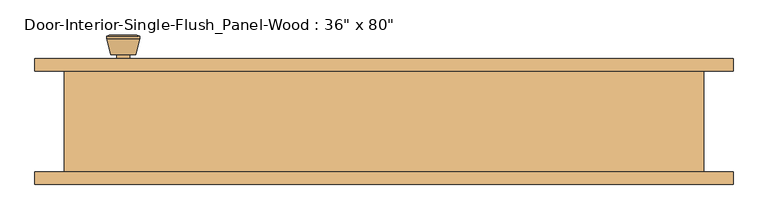
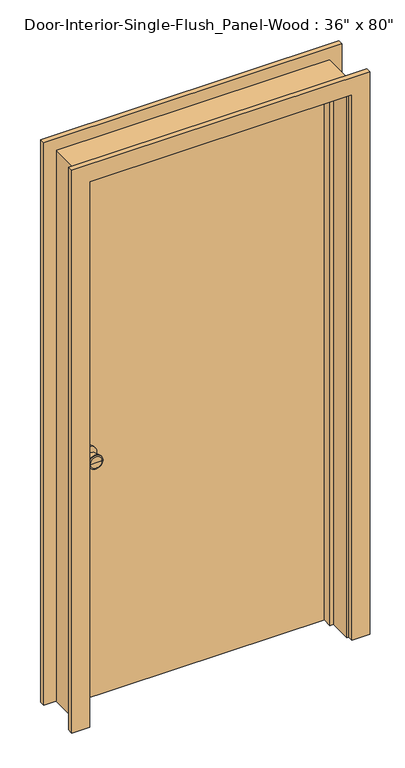
"""IFC4 building model written with IfcOpenShell, lengths in millimetres: door geometry."""

from ifc_helpers import new_model, si_unit, point, frame, frame_2d, origin, origin_with_axes, place, context, project, spatial, polyline, circle_curve, trimmed, segment, composite_curve, outline, extrude, faceted_brep, source, transform, mapped, element, save
from ifc_brep_helpers import plane_surface, cylinder_surface, revolved_surface, advanced_brep


def door_2171c7d8(model_context):
    return source(origin(), model_context, "Body", "SolidModel", [
        advanced_brep(
        [(-393.7, 32.1, 914.4), (-383.7, 32.1, 914.4), (-403.7, 32.1, 914.4), (-373.2241324, -16.9, 914.4), (-393.7, -16.9, 914.4), (-414.1758676, -16.9, 914.4), (-368.7, -15.0721319, 914.4), (-418.7, -15.0721319, 914.4), (-368.7, -11.6084537, 914.4), (-418.7, -11.6084537, 914.4), (-375.063764, 13.1, 914.4), (-412.336236, 13.1, 914.4), (-383.7, 13.1, 914.4), (-403.7, 13.1, 914.4)],
        [
            (0, 1),
            (1, 2, circle_curve(frame((-393.7, 32.1, 914.4), z_axis=(0.0, 1.0, 0.0), x_axis=(-1.0, 0.0, 0.0)), 10.0)),
            (2, 0),
            (2, 1, circle_curve(frame((-393.7, 32.1, 914.4), z_axis=(0.0, 1.0, 0.0), x_axis=(-1.0, 0.0, 0.0)), 10.0)),
            (3, 4),
            (4, 5),
            (5, 3, circle_curve(frame((-393.7, -16.9, 914.4), z_axis=(0.0, -1.0, 0.0), x_axis=(-1.0, 0.0, 0.0)), 20.4758676)),
            (3, 5, circle_curve(frame((-393.7, -16.9, 914.4), z_axis=(0.0, -1.0, 0.0), x_axis=(-1.0, 0.0, 0.0)), 20.4758676)),
            (6, 3),
            (5, 7),
            (7, 6, circle_curve(frame((-393.7, -15.0721319, 914.4), z_axis=(0.0, -1.0, 0.0), x_axis=(-1.0, 0.0, 0.0)), 25.0)),
            (6, 7, circle_curve(frame((-393.7, -15.0721319, 914.4), z_axis=(0.0, -1.0, 0.0), x_axis=(-1.0, 0.0, 0.0)), 25.0)),
            (8, 6),
            (7, 9),
            (9, 8, circle_curve(frame((-393.7, -11.6084537, 914.4), z_axis=(0.0, -1.0, 0.0), x_axis=(-1.0, 0.0, 0.0)), 25.0)),
            (8, 9, circle_curve(frame((-393.7, -11.6084537, 914.4), z_axis=(0.0, -1.0, 0.0), x_axis=(-1.0, 0.0, 0.0)), 25.0)),
            (10, 8),
            (9, 11),
            (11, 10, circle_curve(frame((-393.7, 13.1, 914.4), z_axis=(0.0, -1.0, 0.0), x_axis=(-1.0, 0.0, 0.0)), 18.636236)),
            (10, 11, circle_curve(frame((-393.7, 13.1, 914.4), z_axis=(0.0, -1.0, 0.0), x_axis=(-1.0, 0.0, 0.0)), 18.636236)),
            (12, 10),
            (11, 13),
            (13, 12, circle_curve(frame((-393.7, 13.1, 914.4), z_axis=(0.0, -1.0, 0.0), x_axis=(-1.0, 0.0, 0.0)), 10.0)),
            (12, 13, circle_curve(frame((-393.7, 13.1, 914.4), z_axis=(0.0, -1.0, 0.0), x_axis=(-1.0, 0.0, 0.0)), 10.0)),
            (1, 12),
            (13, 2),
        ],
        [
            plane_surface(frame((-393.7, 32.1, 914.4), z_axis=(0.0, 1.0, 0.0), x_axis=(-1.0, 0.0, 0.0))),
            plane_surface(frame((-393.7, -16.9, 914.4), z_axis=(0.0, -1.0, 0.0), x_axis=(-1.0, 0.0, 0.0))),
            revolved_surface(polyline([(-414.1758676, -16.9, 914.4), (-418.7, -15.0721319, 914.4)]), (-393.7, 32.1, 914.4), (0.0, 1.0, 0.0)),
            cylinder_surface(frame((-393.7, 32.1, 914.4), z_axis=(0.0, 1.0, 0.0), x_axis=(-1.0, 0.0, 0.0)), 25.0),
            revolved_surface(polyline([(-418.7, -11.6084537, 914.4), (-412.336236, 13.1, 914.4)]), (-393.7, 32.1, 914.4), (0.0, 1.0, 0.0)),
            plane_surface(frame((-393.7, 13.1, 914.4), z_axis=(0.0, 1.0, 0.0), x_axis=(-1.0, 0.0, 0.0))),
            cylinder_surface(frame((-393.7, 32.1, 914.4), z_axis=(0.0, 1.0, 0.0), x_axis=(-1.0, 0.0, 0.0)), 10.0),
        ],
        [
            (0, [[1, 2, 3]]),
            (0, [[-3, 4, -1]]),
            (1, [[5, 6, 7]]),
            (1, [[-6, -5, 8]]),
            (2, [[9, -7, 10, 11]]),
            (2, [[-10, -8, -9, 12]]),
            (3, [[13, -11, 14, 15]]),
            (3, [[-14, -12, -13, 16]]),
            (4, [[17, -15, 18, 19]]),
            (4, [[-18, -16, -17, 20]]),
            (5, [[21, -19, 22, 23]]),
            (5, [[-22, -20, -21, 24]]),
            (6, [[25, -23, 26, -2]]),
            (6, [[-26, -24, -25, -4]]),
        ],
    ),
        extrude(outline(composite_curve([segment(trimmed(circle_curve(frame_2d((914.4, -393.7)), 30.0), [point((914.4, -423.7))], [point((914.4, -363.7))], False, "CARTESIAN"), True, "CONTINUOUS"), segment(trimmed(circle_curve(frame_2d((914.4, -393.7)), 30.0), [point((914.4, -363.7))], [point((914.4, -423.7))], False, "CARTESIAN"), True, "CONTINUOUS")], self_intersect=False)), frame((0.0, 32.1, 0.0), z_axis=(0.0, 1.0, 0.0), x_axis=(0.0, 0.0, 1.0)), (0.0, 0.0, 1.0), 6.0),
        advanced_brep(
        [(-393.7, 79.025, 914.4), (-403.7, 79.025, 914.4), (-383.7, 79.025, 914.4), (-373.2241324, 128.025, 914.4), (-414.1758676, 128.025, 914.4), (-393.7, 128.025, 914.4), (-368.7, 126.1971319, 914.4), (-418.7, 126.1971319, 914.4), (-368.7, 122.7334537, 914.4), (-418.7, 122.7334537, 914.4), (-375.063764, 98.025, 914.4), (-412.336236, 98.025, 914.4), (-383.7, 98.025, 914.4), (-403.7, 98.025, 914.4)],
        [
            (0, 1),
            (1, 2, circle_curve(frame((-393.7, 79.025, 914.4), z_axis=(0.0, -1.0, 0.0), x_axis=(-1.0, 0.0, 0.0)), 10.0)),
            (2, 0),
            (2, 1, circle_curve(frame((-393.7, 79.025, 914.4), z_axis=(0.0, -1.0, 0.0), x_axis=(-1.0, 0.0, 0.0)), 10.0)),
            (3, 4, circle_curve(frame((-393.7, 128.025, 914.4), z_axis=(0.0, 1.0, 0.0), x_axis=(-1.0, 0.0, 0.0)), 20.4758676)),
            (4, 5),
            (5, 3),
            (4, 3, circle_curve(frame((-393.7, 128.025, 914.4), z_axis=(0.0, 1.0, 0.0), x_axis=(-1.0, 0.0, 0.0)), 20.4758676)),
            (6, 7, circle_curve(frame((-393.7, 126.1971319, 914.4), z_axis=(0.0, 1.0, 0.0), x_axis=(-1.0, 0.0, 0.0)), 25.0)),
            (7, 4),
            (3, 6),
            (7, 6, circle_curve(frame((-393.7, 126.1971319, 914.4), z_axis=(0.0, 1.0, 0.0), x_axis=(-1.0, 0.0, 0.0)), 25.0)),
            (8, 9, circle_curve(frame((-393.7, 122.7334537, 914.4), z_axis=(0.0, 1.0, 0.0), x_axis=(-1.0, 0.0, 0.0)), 25.0)),
            (9, 7),
            (6, 8),
            (9, 8, circle_curve(frame((-393.7, 122.7334537, 914.4), z_axis=(0.0, 1.0, 0.0), x_axis=(-1.0, 0.0, 0.0)), 25.0)),
            (10, 11, circle_curve(frame((-393.7, 98.025, 914.4), z_axis=(0.0, 1.0, 0.0), x_axis=(-1.0, 0.0, 0.0)), 18.636236)),
            (11, 9),
            (8, 10),
            (11, 10, circle_curve(frame((-393.7, 98.025, 914.4), z_axis=(0.0, 1.0, 0.0), x_axis=(-1.0, 0.0, 0.0)), 18.636236)),
            (12, 13, circle_curve(frame((-393.7, 98.025, 914.4), z_axis=(0.0, 1.0, 0.0), x_axis=(-1.0, 0.0, 0.0)), 10.0)),
            (13, 11),
            (10, 12),
            (13, 12, circle_curve(frame((-393.7, 98.025, 914.4), z_axis=(0.0, 1.0, 0.0), x_axis=(-1.0, 0.0, 0.0)), 10.0)),
            (1, 13),
            (12, 2),
        ],
        [
            plane_surface(frame((-393.7, 79.025, 914.4), z_axis=(0.0, -1.0, 0.0), x_axis=(-1.0, 0.0, 0.0))),
            plane_surface(frame((-393.7, 128.025, 914.4), z_axis=(0.0, 1.0, 0.0), x_axis=(-1.0, 0.0, 0.0))),
            revolved_surface(polyline([(-414.1758676, 128.025, 914.4), (-418.7, 126.1971319, 914.4)]), (-393.7, 79.025, 914.4), (0.0, -1.0, 0.0)),
            cylinder_surface(frame((-393.7, 79.025, 914.4), z_axis=(0.0, -1.0, 0.0), x_axis=(-1.0, 0.0, 0.0)), 25.0),
            revolved_surface(polyline([(-418.7, 122.7334537, 914.4), (-412.336236, 98.025, 914.4)]), (-393.7, 79.025, 914.4), (0.0, -1.0, 0.0)),
            plane_surface(frame((-393.7, 98.025, 914.4), z_axis=(0.0, -1.0, 0.0), x_axis=(-1.0, 0.0, 0.0))),
            cylinder_surface(frame((-393.7, 79.025, 914.4), z_axis=(0.0, -1.0, 0.0), x_axis=(-1.0, 0.0, 0.0)), 10.0),
        ],
        [
            (0, [[1, 2, 3]]),
            (0, [[-3, 4, -1]]),
            (1, [[5, 6, 7]]),
            (1, [[8, -7, -6]]),
            (2, [[9, 10, -5, 11]]),
            (2, [[12, -11, -8, -10]]),
            (3, [[13, 14, -9, 15]]),
            (3, [[16, -15, -12, -14]]),
            (4, [[17, 18, -13, 19]]),
            (4, [[20, -19, -16, -18]]),
            (5, [[21, 22, -17, 23]]),
            (5, [[24, -23, -20, -22]]),
            (6, [[-2, 25, -21, 26]]),
            (6, [[-4, -26, -24, -25]]),
        ],
    ),
        extrude(outline(composite_curve([segment(trimmed(circle_curve(frame_2d((914.4, -393.7)), 30.0), [point((914.4, -423.7))], [point((914.4, -363.7))], False, "CARTESIAN"), True, "CONTINUOUS"), segment(trimmed(circle_curve(frame_2d((914.4, -393.7)), 30.0), [point((914.4, -363.7))], [point((914.4, -423.7))], False, "CARTESIAN"), True, "CONTINUOUS")], self_intersect=False)), frame((0.0, 73.025, 0.0), z_axis=(0.0, 1.0, 0.0), x_axis=(0.0, 0.0, 1.0)), (0.0, 0.0, 1.0), 6.0),
        extrude(outline(polyline([(457.2, 38.1), (-457.2, 38.1), (-457.2, 73.025), (457.2, 73.025), (457.2, 38.1)])), origin_with_axes(), (0.0, 0.0, 1.0), 2032.0),
        faceted_brep([(482.6, 73.025, 0.0), (482.6, -79.375, 0.0), (457.2, -79.375, 0.0), (457.2, 3.175, 0.0), (444.5, 3.175, 0.0), (444.5, 38.1, 0.0), (457.2, 38.1, 0.0), (457.2, 73.025, 0.0), (482.6, 73.025, 2057.4), (482.6, -79.375, 2057.4), (-482.6, -79.375, 2057.4), (-482.6, -79.375, 0.0), (-457.2, -79.375, 0.0), (-457.2, -79.375, 2032.0), (457.2, -79.375, 2032.0), (457.2, 3.175, 2032.0), (-457.2, 3.175, 2032.0), (-457.2, 3.175, 0.0), (-444.5, 3.175, 0.0), (-444.5, 3.175, 2019.3), (444.5, 3.175, 2019.3), (444.5, 38.1, 2019.3), (-444.5, 38.1, 2019.3), (-444.5, 38.1, 0.0), (-457.2, 38.1, 0.0), (-457.2, 38.1, 2032.0), (457.2, 38.1, 2032.0), (457.2, 73.025, 2032.0), (-457.2, 73.025, 2032.0), (-457.2, 73.025, 0.0), (-482.6, 73.025, 0.0), (-482.6, 73.025, 2057.4)], [[[0, 1, 2, 3, 4, 5, 6, 7]], [[1, 0, 8, 9]], [[2, 1, 9, 10, 11, 12, 13, 14]], [[3, 2, 14, 15]], [[4, 3, 15, 16, 17, 18, 19, 20]], [[5, 4, 20, 21]], [[6, 5, 21, 22, 23, 24, 25, 26]], [[7, 6, 26, 27]], [[0, 7, 27, 28, 29, 30, 31, 8]], [[9, 8, 31, 10]], [[15, 14, 13, 16]], [[21, 20, 19, 22]], [[27, 26, 25, 28]], [[30, 29, 24, 23, 18, 17, 12, 11]], [[10, 31, 30, 11]], [[16, 13, 12, 17]], [[22, 19, 18, 23]], [[28, 25, 24, 29]]]),
        extrude(outline(polyline([(0.0, 463.55), (0.0, 527.05), (2101.85, 527.05), (2101.85, -527.05), (0.0, -527.05), (0.0, -463.55), (2038.35, -463.55), (2038.35, 463.55), (0.0, 463.55)])), frame((0.0, -98.425, 0.0), z_axis=(0.0, 1.0, 0.0), x_axis=(0.0, 0.0, 1.0)), (0.0, 0.0, 1.0), 19.05),
        extrude(outline(polyline([(0.0, 463.55), (0.0, 527.05), (2101.85, 527.05), (2101.85, -527.05), (0.0, -527.05), (0.0, -463.55), (2038.35, -463.55), (2038.35, 463.55), (0.0, 463.55)])), frame((0.0, 73.025, 0.0), z_axis=(0.0, 1.0, 0.0), x_axis=(0.0, 0.0, 1.0)), (0.0, 0.0, 1.0), 19.05),
    ])


if __name__ == "__main__":
    model = new_model("IFC4")
    model_context = context("Model", 3, world=origin())
    ifc_project = project(units=[si_unit("LENGTHUNIT", "METRE", prefix="MILLI")], contexts=[model_context])
    site = spatial("IfcSite", under=ifc_project)
    building = spatial("IfcBuilding", under=site)
    placement = place(None, origin())
    door_shape = door_2171c7d8(model_context)
    element("IfcDoor", 1, ObjectType="Door-Interior-Single-Flush_Panel-Wood : 36\" x 80\"", at=placement, inside=building, context=model_context, shape_type="MappedRepresentation", body=[
        mapped(door_shape, transform((0.0, 0.0, 0.0), x_axis=(1.0, 0.0, 0.0), y_axis=(0.0, 1.0, 0.0), z_axis=(0.0, 0.0, 1.0))),
    ])
    save(model, "model.ifc")

# Revit data of these elements
# Type "Door-Interior-Single-Flush_Panel-Wood : 36\" x 80\""
#   Type Mark = "9"
#   Assembly Code = "C1020300"
#   Analytic Construction = "Wooden"
#   Thickness = 0' - 1 3/8"
#   Thermal Resistance (R) = 2.5876 (h·ft²·°F)/BTU
#   Swing Angle [instance default] = 90.00°
#   Rough Width = 3' - 2"
#   Rough Height = 6' - 9"
#   Height = 6' - 8"
#   Width = 3' - 0"
#   Heat Transfer Coefficient (U) = 0.3865 BTU/(h·ft²·°F)
#   Trim Material = Cherry
#   Panel Material = Cherry
#   Frame Material = Cherry
#   Door Handle Material = Aluminum
#   Visual Light Transmittance = 0
#   Solar Heat Gain Coefficient = 0
#   Wall Closure = (empty or 0)
#   Function = (empty or 0)
# Element 1 (IfcDoor, "Door-Interior-Single-Flush_Panel-Wood : 36\" x 80\"")
#   Materials on its faces: "Cherry", "Aluminum"
# Materials
#   "Cherry": class "Wood", colour RGB 226 177 128, transparency 0, Description = "Prunus Serotina", Cost = 0
#   "Aluminum": class "Metal", colour RGB 247 247 247, transparency 0, Description = "Aluminum 6061", Cost = 0
